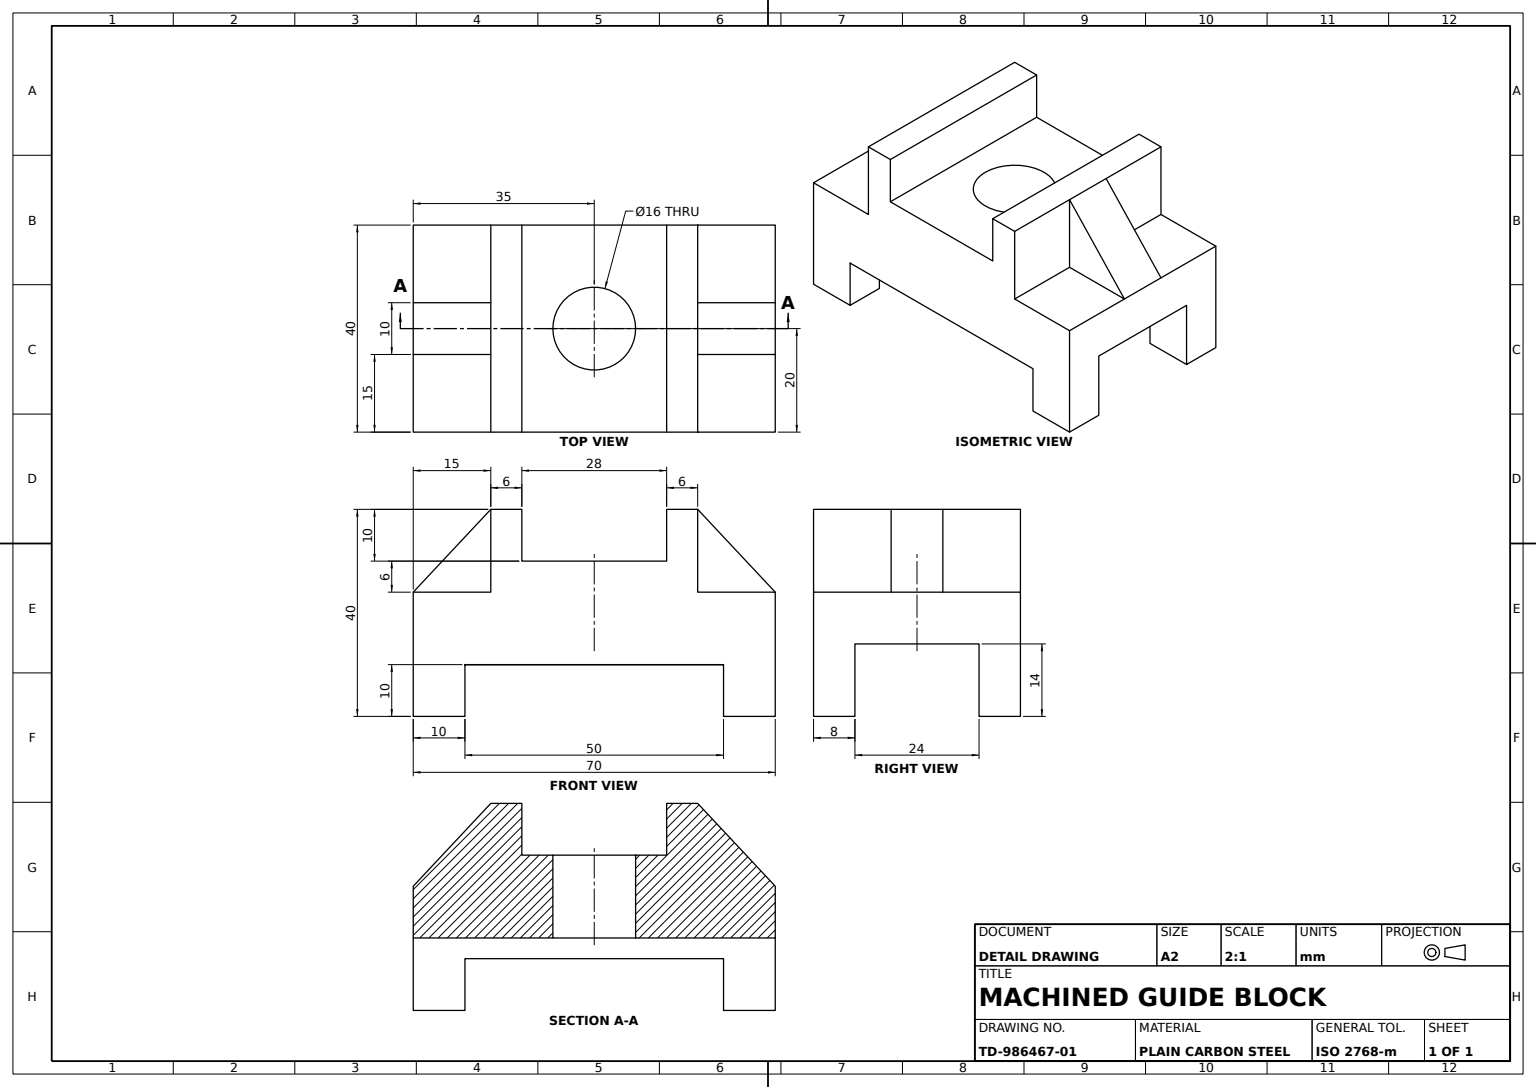
from build123d import *

# Parameters (mm, degrees)
BASE_BLOCK_70X40X40_DEPTH        = 40
BOTTOM_SLOT_SKETCH_W             = 24
BOTTOM_SLOT_SKETCH_H             = 14
BOTTOM_SLOT_DEPTH                = 35
BOTTOM_SLOT_EXTENSION_SKETCH_W   = 24
BOTTOM_SLOT_EXTENSION_SKETCH_H   = 14
BOTTOM_SLOT_EXTENSION_DEPTH      = 35
TOP_CHANNEL_SKETCH_W             = 14
TOP_CHANNEL_SKETCH_H             = 10
TOP_CHANNEL_DEPTH                = 49
SIDE_STEP_CUT_A_DEPTH            = 67.520673478
SIDE_STEP_CUT_A_DEPTH_BACK       = 95
SIDE_STEP_CUT_A_SKETCH_W         = 15
SIDE_STEP_CUT_A_SKETCH_H         = 16
SIDE_STEP_CUT_B_SKETCH_W         = 15
SIDE_STEP_CUT_B_SKETCH_H         = 16
SIDE_STEP_CUT_B_DEPTH            = 95
RIB_A_SKETCH_W                   = 15
RIB_A_SKETCH_H                   = 5
RIB_A_DEPTH                      = 16
RIB_A_TRIM_DEPTH                 = 40
RIB_A_TRIM_DEPTH_BACK            = 52
THROUGH_HOLE_16_DEPTH            = 52
THROUGH_HOLE_16_DEPTH_BACK       = 52
THROUGH_HOLE_16_SKETCH_R         = 8
RIB_B_SKETCH_W                   = 15
RIB_B_SKETCH_H                   = 5
RIB_B_DEPTH                      = 16
RIB_B_TRIM_DEPTH                 = 16
FOOT_RELIEF_CUT_DEPTH            = 23
FOOT_RELIEF_CUT_DEPTH_BACK       = 23
FOOT_RELIEF_SKETCH_W             = 50
FOOT_RELIEF_SKETCH_H             = 10
FOOT_RELIEF_EXTENSION_DEPTH      = 23
FOOT_RELIEF_EXTENSION_DEPTH_BACK = 23
FOOT_RELIEF_EXTENSION_SKETCH_W   = 50
FOOT_RELIEF_EXTENSION_SKETCH_H   = 10


with BuildPart() as part:
    # Base Block Sketch → Base Block 70x40x40 (new body)
    with BuildSketch(Plane(origin=(0, 0, 0), x_dir=(1, 0, 0), z_dir=(0, 1, 0))):
        Polygon((0, -20), (0, 0), (0, 20), (-35, 20), (-35, -20), align=None)
        Polygon((0, 20), (0, 0), (0, -20), (35, -20), (35, 20), align=None)
    extrude(amount=BASE_BLOCK_70X40X40_DEPTH)

    # Bottom Slot Sketch → Bottom Slot (cut)
    with BuildSketch(Plane.ZY.offset(35)):
        with Locations((0, 7)):
            Rectangle(BOTTOM_SLOT_SKETCH_W, BOTTOM_SLOT_SKETCH_H)
    extrude(amount=-BOTTOM_SLOT_DEPTH, mode=Mode.SUBTRACT)

    # Bottom Slot Extension Sketch → Bottom Slot Extension (cut)
    with BuildSketch(Plane.ZY):
        with Locations((0, 7)):
            Rectangle(BOTTOM_SLOT_EXTENSION_SKETCH_W, BOTTOM_SLOT_EXTENSION_SKETCH_H)
    extrude(amount=-BOTTOM_SLOT_EXTENSION_DEPTH, mode=Mode.SUBTRACT)

    # Top Channel Sketch → Top Channel (cut)
    with BuildSketch(Plane.XY.offset(20)):
        with Locations((-7, 35)):
            Rectangle(TOP_CHANNEL_SKETCH_W, TOP_CHANNEL_SKETCH_H)
        with Locations((7, 35)):
            Rectangle(TOP_CHANNEL_SKETCH_W, TOP_CHANNEL_SKETCH_H)
    extrude(amount=-TOP_CHANNEL_DEPTH, mode=Mode.SUBTRACT)

    # Side Step Cut A Sketch → Side Step Cut A (cut, two sides: drawn at the far end of the back side and taken through both)
    with BuildSketch(Plane.XY.offset(20).offset(-SIDE_STEP_CUT_A_DEPTH_BACK)):
        with Locations((27.5, 32)):
            Rectangle(SIDE_STEP_CUT_A_SKETCH_W, SIDE_STEP_CUT_A_SKETCH_H)
    extrude(amount=SIDE_STEP_CUT_A_DEPTH + SIDE_STEP_CUT_A_DEPTH_BACK, mode=Mode.SUBTRACT)

    # Side Step Cut B Sketch → Side Step Cut B (cut)
    with BuildSketch(Plane.XY.offset(20)):
        with Locations((-27.5, 32)):
            Rectangle(SIDE_STEP_CUT_B_SKETCH_W, SIDE_STEP_CUT_B_SKETCH_H)
    extrude(amount=-SIDE_STEP_CUT_B_DEPTH, mode=Mode.SUBTRACT)

    # Rib A Sketch → Rib A (add)
    with BuildSketch(Plane(origin=(0, 24, 0), x_dir=(1, 0, 0), z_dir=(0, 1, 0))):
        with Locations((-27.5, -2.5)):
            Rectangle(RIB_A_SKETCH_W, RIB_A_SKETCH_H)
        with Locations((-27.5, 2.5)):
            Rectangle(RIB_A_SKETCH_W, RIB_A_SKETCH_H)
    extrude(amount=RIB_A_DEPTH)

    # Rib A Trim Sketch → Rib A Trim (cut, two sides: drawn at the far end of the back side and taken through both)
    with BuildSketch(Plane.XY.offset(5).offset(-RIB_A_TRIM_DEPTH_BACK)):
        Polygon((-20, 40), (-35, 24), (-35, 40), align=None)
    extrude(amount=RIB_A_TRIM_DEPTH + RIB_A_TRIM_DEPTH_BACK, mode=Mode.SUBTRACT)

    # Through Hole _16 Sketch → Through Hole _16 (cut, two sides: drawn at the far end of the back side and taken through both)
    with BuildSketch(Plane(origin=(0, 30, 0), x_dir=(1, 0, 0), z_dir=(0, 1, 0)).offset(-THROUGH_HOLE_16_DEPTH_BACK)):
        with Locations(Location((0, 0, 0), (0, 0, 270))):
            Circle(THROUGH_HOLE_16_SKETCH_R)
    extrude(amount=THROUGH_HOLE_16_DEPTH + THROUGH_HOLE_16_DEPTH_BACK, mode=Mode.SUBTRACT)

    # Rib B Sketch → Rib B (add)
    with BuildSketch(Plane(origin=(0, 24, 0), x_dir=(1, 0, 0), z_dir=(0, 1, 0))):
        with Locations((27.5, -2.5)):
            Rectangle(RIB_B_SKETCH_W, RIB_B_SKETCH_H)
        with Locations((27.5, 2.5)):
            Rectangle(RIB_B_SKETCH_W, RIB_B_SKETCH_H)
    extrude(amount=RIB_B_DEPTH)

    # Rib B Trim Sketch → Rib B Trim (cut)
    with BuildSketch(Plane(origin=(0, 0, -5), x_dir=(-1, 0, 0), z_dir=(0, 0, -1))):
        Polygon((-20, 40), (-35, 24), (-35, 40), align=None)
    extrude(amount=-RIB_B_TRIM_DEPTH, mode=Mode.SUBTRACT)

    # Foot Relief Sketch → Foot Relief Cut (cut, two sides: drawn at the far end of the back side and taken through both)
    with BuildSketch(Plane(origin=(0, 0, -20), x_dir=(-1, 0, 0), z_dir=(0, 0, -1)).offset(-FOOT_RELIEF_CUT_DEPTH_BACK)):
        with Locations((0, 5)):
            Rectangle(FOOT_RELIEF_SKETCH_W, FOOT_RELIEF_SKETCH_H)
    extrude(amount=FOOT_RELIEF_CUT_DEPTH + FOOT_RELIEF_CUT_DEPTH_BACK, mode=Mode.SUBTRACT)

    # Foot Relief Extension Sketch → Foot Relief Extension (cut, two sides: drawn at the far end of the back side and taken through both)
    with BuildSketch(Plane(origin=(0, 0, 12), x_dir=(-1, 0, 0), z_dir=(0, 0, -1)).offset(-FOOT_RELIEF_EXTENSION_DEPTH_BACK)):
        with Locations((0, 5)):
            Rectangle(FOOT_RELIEF_EXTENSION_SKETCH_W, FOOT_RELIEF_EXTENSION_SKETCH_H)
    extrude(amount=FOOT_RELIEF_EXTENSION_DEPTH + FOOT_RELIEF_EXTENSION_DEPTH_BACK, mode=Mode.SUBTRACT)


solid = part.part
